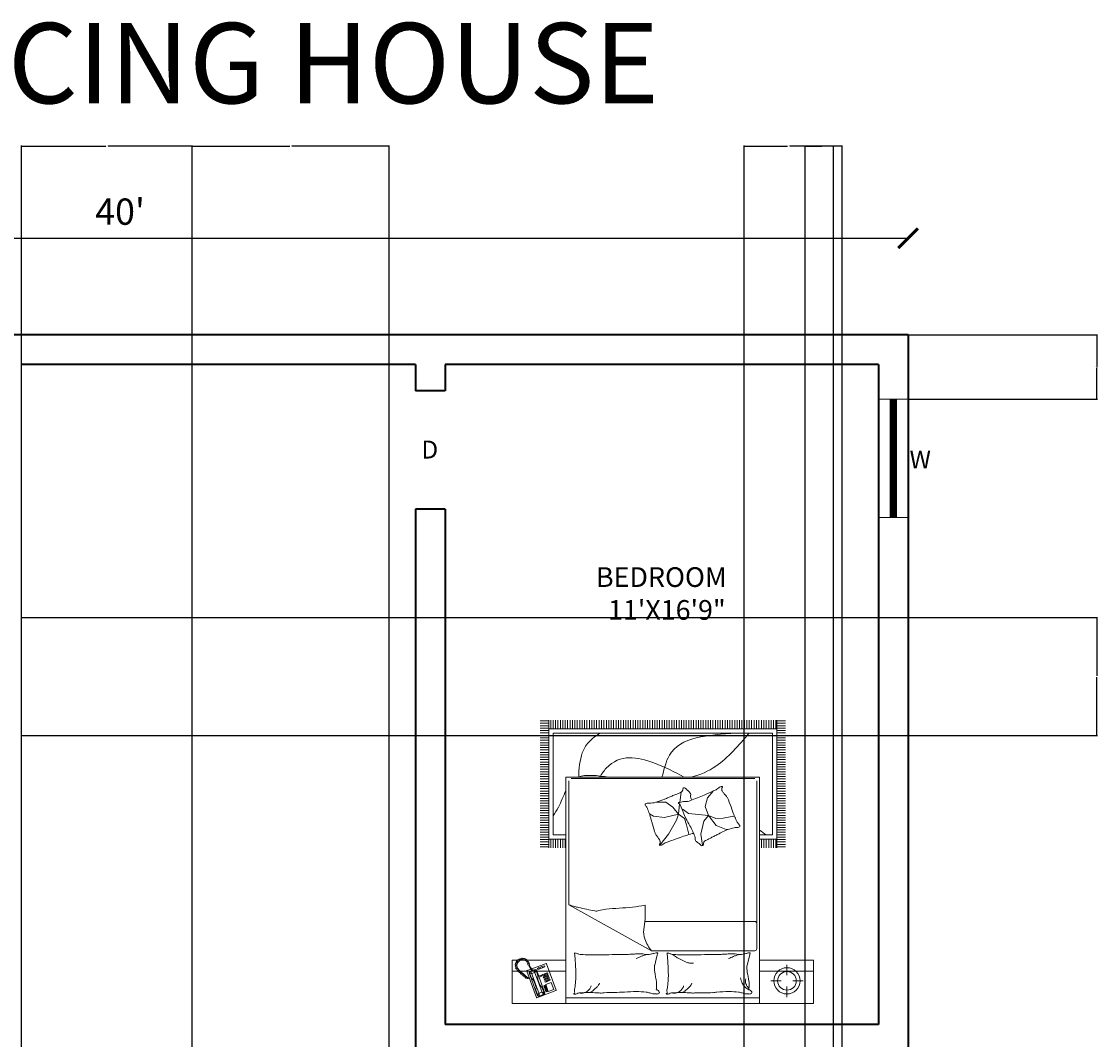
# Model space of a CAD drawing. Units: inches. Extents: x 318 to 927, y -1130 to 13.
# Tile 17 of 17: x 599 to 927, y -297 to 13. Entities that reach past the tile are written whole.
import ezdxf

# ---------------------------------------------------------------- set-up
doc = ezdxf.new("R2010")
doc.units = ezdxf.units.IN
doc.header["$MEASUREMENT"] = 0
for name, color, linetype, lineweight in [('A-ANNO-DIMS', 1, 'Continuous', 18), ('A-ANNO-IDEN', 1, 'Continuous', 13), ('A-ANNO-TEXT', 8, 'Continuous', 25), ('A-AREA-IDEN', 8, 'Continuous', 18), ('A-GLAZ-PATT', 5, 'Continuous', 9), ('wall', 1, 'Continuous', 35), ('win', 5, 'Continuous', 18)]:
    doc.layers.add(name, color=color, linetype=linetype, lineweight=lineweight)
doc.layers.add('furniture', color=50, linetype='Continuous', lineweight=13, transparency=0.8)
doc.styles.add('DIM_FONT', font='SIMPLEX.shx', dxfattribs={"width": 0.8})
doc.styles.get("Standard").update_dxf_attribs({"font": 'arial.ttf'})
doc.dimstyles.get("Standard").update_dxf_attribs({"dimtxt": 0.18, "dimasz": 0.18, "dimexe": 0.18, "dimexo": 0.0625, "dimgap": 0.09, "dimtad": 0, "dimtih": 1, "dimtoh": 1, "dimdec": 1, "dimzin": 0, "dimdsep": 46, "dimlunit": 4, "dimtxsty": 'Standard', "dimcen": 0.09, "dimadec": 0, "dimazin": 0, "dimtfac": 1, "dimtdec": 1, "dimtofl": 0, "dimtmove": 0, "dimatfit": 3, "dimfxl": 1, "dimtolj": 1, "dimtzin": 0, "dimarcsym": 0})

# ---------------------------------------------------------------- blocks, each defined once
blk = doc.blocks.new('A$C4F634EDD')
for p, q in [((0, 2.629), (0, 2.229)), ((0.5, 2.629), (0, 2.629)), ((0.5, 2.629), (2.3, 2.629)), ((0.5, 0.529), (0.5, 2.629)), ((0.5, 2.229), (0.5, 2.629)), ((2.3, 2.629), (2.3, 0.529)), ((2.3, 2.629), (2.8, 2.629)), ((2.3, 2.229), (2.3, 2.629)), ((2.8, 2.629), (2.8, 2.229)), ((0.246, 2.57), (0.246, 2.473)), ((0.5, 2.577), (2.3, 2.577)), ((2.39, 2.507), (2.392, 2.511)), ((2.48, 2.262), (2.39, 2.507)), ((2.392, 2.511), (2.569, 2.577)), ((2.412, 2.501), (2.463, 2.52)), ((2.463, 2.52), (2.487, 2.454)), ((2.484, 2.523), (2.47, 2.518)), ((2.47, 2.518), (2.472, 2.513)), ((2.472, 2.513), (2.486, 2.518)), ((2.488, 2.513), (2.474, 2.507)), ((2.474, 2.507), (2.476, 2.502)), ((2.476, 2.502), (2.49, 2.507)), ((2.492, 2.502), (2.478, 2.497)), ((2.486, 2.518), (2.484, 2.523)), ((2.49, 2.507), (2.488, 2.513)), ((2.494, 2.497), (2.492, 2.502)), ((2.495, 2.533), (2.498, 2.545)), ((2.573, 2.319), (2.495, 2.533)), ((2.498, 2.545), (2.552, 2.564)), ((2.506, 2.545), (2.5, 2.539)), ((2.5, 2.539), (2.501, 2.531)), ((2.501, 2.531), (2.519, 2.484)), ((2.501, 2.531), (2.523, 2.521)), ((2.506, 2.545), (2.549, 2.561)), ((2.524, 2.526), (2.506, 2.545)), ((2.523, 2.521), (2.524, 2.526)), ((2.552, 2.442), (2.523, 2.521)), ((2.548, 2.535), (2.524, 2.526)), ((2.548, 2.535), (2.549, 2.561)), ((2.551, 2.532), (2.548, 2.535)), ((2.549, 2.561), (2.557, 2.56)), ((2.562, 2.554), (2.551, 2.532)), ((2.581, 2.452), (2.551, 2.532)), ((2.552, 2.564), (2.564, 2.558)), ((2.557, 2.56), (2.562, 2.554)), ((2.562, 2.554), (2.579, 2.506)), ((2.564, 2.558), (2.642, 2.346)), ((2.569, 2.577), (2.574, 2.574)), ((2.574, 2.574), (2.664, 2.33)), ((2.579, 2.506), (2.579, 2.496)), ((0.096, 2.42), (0.192, 2.42)), ((0.299, 2.42), (0.396, 2.42)), ((2.436, 2.435), (2.412, 2.501)), ((2.487, 2.454), (2.436, 2.435)), ((2.446, 2.415), (2.456, 2.418)), ((2.45, 2.404), (2.446, 2.415)), ((2.46, 2.408), (2.45, 2.404)), ((2.456, 2.418), (2.46, 2.408)), ((2.463, 2.421), (2.474, 2.425)), ((2.467, 2.41), (2.463, 2.421)), ((2.478, 2.414), (2.467, 2.41)), ((2.471, 2.402), (2.481, 2.405)), ((2.474, 2.391), (2.471, 2.402)), ((2.474, 2.425), (2.478, 2.414)), ((2.478, 2.497), (2.48, 2.491)), ((2.48, 2.491), (2.494, 2.497)), ((2.481, 2.428), (2.492, 2.431)), ((2.485, 2.417), (2.481, 2.428)), ((2.481, 2.405), (2.485, 2.395)), ((2.496, 2.491), (2.482, 2.486)), ((2.482, 2.486), (2.484, 2.481)), ((2.484, 2.481), (2.498, 2.486)), ((2.496, 2.421), (2.485, 2.417)), ((2.5, 2.481), (2.486, 2.475)), ((2.486, 2.475), (2.488, 2.47)), ((2.488, 2.47), (2.502, 2.475)), ((2.488, 2.408), (2.499, 2.412)), ((2.492, 2.397), (2.488, 2.408)), ((2.504, 2.47), (2.49, 2.465)), ((2.49, 2.465), (2.491, 2.46)), ((2.491, 2.46), (2.506, 2.465)), ((2.492, 2.431), (2.496, 2.421)), ((2.503, 2.401), (2.492, 2.397)), ((2.498, 2.486), (2.496, 2.491)), ((2.499, 2.412), (2.503, 2.401)), ((2.502, 2.475), (2.5, 2.481)), ((2.506, 2.465), (2.504, 2.47)), ((2.519, 2.484), (2.526, 2.476)), ((2.526, 2.476), (2.534, 2.469)), ((2.534, 2.469), (2.541, 2.457)), ((2.541, 2.457), (2.547, 2.44)), ((2.559, 2.406), (2.547, 2.44)), ((2.552, 2.442), (2.587, 2.346)), ((2.562, 2.393), (2.559, 2.406)), ((2.579, 2.496), (2.577, 2.485)), ((2.577, 2.485), (2.579, 2.472)), ((2.579, 2.472), (2.586, 2.454)), ((2.581, 2.452), (2.616, 2.356)), ((2.598, 2.42), (2.586, 2.454)), ((2.605, 2.409), (2.598, 2.42)), ((2.613, 2.402), (2.605, 2.409)), ((2.62, 2.394), (2.613, 2.402)), ((0, 2.33), (0.5, 2.33)), ((0.246, 2.366), (0.246, 2.27)), ((2.8, 2.33), (2.3, 2.33)), ((2.453, 2.395), (2.463, 2.399)), ((2.457, 2.384), (2.453, 2.395)), ((2.467, 2.388), (2.457, 2.384)), ((2.46, 2.376), (2.471, 2.379)), ((2.464, 2.365), (2.46, 2.376)), ((2.463, 2.399), (2.467, 2.388)), ((2.475, 2.369), (2.464, 2.365)), ((2.467, 2.356), (2.478, 2.36)), ((2.471, 2.345), (2.467, 2.356)), ((2.471, 2.379), (2.475, 2.369)), ((2.482, 2.349), (2.471, 2.345)), ((2.485, 2.395), (2.474, 2.391)), ((2.478, 2.382), (2.488, 2.386)), ((2.482, 2.371), (2.478, 2.382)), ((2.478, 2.36), (2.482, 2.349)), ((2.492, 2.375), (2.482, 2.371)), ((2.617, 2.309), (2.484, 2.26)), ((2.485, 2.363), (2.495, 2.367)), ((2.489, 2.352), (2.485, 2.363)), ((2.488, 2.386), (2.492, 2.375)), ((2.499, 2.356), (2.489, 2.352)), ((2.495, 2.389), (2.506, 2.392)), ((2.499, 2.378), (2.495, 2.389)), ((2.495, 2.367), (2.499, 2.356)), ((2.51, 2.382), (2.499, 2.378)), ((2.503, 2.369), (2.513, 2.373)), ((2.506, 2.358), (2.503, 2.369)), ((2.506, 2.392), (2.51, 2.382)), ((2.517, 2.362), (2.506, 2.358)), ((2.513, 2.373), (2.517, 2.362)), ((2.536, 2.305), (2.518, 2.299)), ((2.524, 2.377), (2.538, 2.382)), ((2.528, 2.366), (2.524, 2.377)), ((2.542, 2.371), (2.528, 2.366)), ((2.54, 2.294), (2.536, 2.305)), ((2.538, 2.382), (2.542, 2.371)), ((2.561, 2.314), (2.543, 2.308)), ((2.543, 2.308), (2.547, 2.297)), ((2.547, 2.297), (2.565, 2.304)), ((2.56, 2.382), (2.562, 2.393)), ((2.56, 2.372), (2.56, 2.382)), ((2.577, 2.324), (2.56, 2.372)), ((2.565, 2.304), (2.561, 2.314)), ((2.585, 2.313), (2.573, 2.319)), ((2.577, 2.324), (2.587, 2.346)), ((2.582, 2.318), (2.577, 2.324)), ((2.59, 2.317), (2.582, 2.318)), ((2.61, 2.322), (2.585, 2.313)), ((2.587, 2.346), (2.591, 2.343)), ((2.591, 2.343), (2.59, 2.317)), ((2.59, 2.317), (2.61, 2.324)), ((2.615, 2.352), (2.591, 2.343)), ((2.613, 2.331), (2.608, 2.329)), ((2.608, 2.329), (2.614, 2.314)), ((2.619, 2.317), (2.613, 2.331)), ((2.614, 2.314), (2.624, 2.298)), ((2.616, 2.356), (2.615, 2.352)), ((2.615, 2.352), (2.633, 2.332)), ((2.615, 2.326), (2.633, 2.332)), ((2.638, 2.346), (2.616, 2.356)), ((2.637, 2.332), (2.616, 2.324)), ((2.626, 2.307), (2.619, 2.317)), ((2.638, 2.346), (2.62, 2.394)), ((2.662, 2.325), (2.623, 2.311)), ((2.636, 2.292), (2.626, 2.307)), ((2.633, 2.332), (2.638, 2.339)), ((2.642, 2.346), (2.637, 2.332)), ((2.638, 2.339), (2.638, 2.346)), ((2.65, 2.398), (2.64, 2.395)), ((2.642, 2.39), (2.649, 2.391)), ((2.649, 2.391), (2.654, 2.39)), ((2.655, 2.397), (2.65, 2.398)), ((2.654, 2.39), (2.66, 2.388)), ((2.663, 2.392), (2.655, 2.397)), ((2.66, 2.388), (2.663, 2.387)), ((2.664, 2.33), (2.662, 2.325)), ((2.669, 2.394), (2.663, 2.392)), ((2.663, 2.387), (2.666, 2.388)), ((2.666, 2.388), (2.663, 2.383)), ((2.663, 2.383), (2.674, 2.374)), ((2.674, 2.394), (2.669, 2.394)), ((2.676, 2.391), (2.674, 2.394)), ((2.674, 2.38), (2.676, 2.391)), ((2.682, 2.386), (2.674, 2.38)), ((2.674, 2.374), (2.692, 2.359)), ((2.687, 2.381), (2.682, 2.386)), ((2.685, 2.369), (2.687, 2.381)), ((2.695, 2.376), (2.685, 2.369)), ((2.692, 2.359), (2.705, 2.347)), ((2.7, 2.371), (2.695, 2.376)), ((2.695, 2.36), (2.7, 2.371)), ((2.703, 2.368), (2.695, 2.36)), ((2.71, 2.362), (2.703, 2.368)), ((2.705, 2.347), (2.708, 2.348)), ((2.706, 2.351), (2.71, 2.362)), ((2.715, 2.358), (2.706, 2.351)), ((2.708, 2.348), (2.708, 2.344)), ((2.708, 2.344), (2.727, 2.328)), ((2.721, 2.352), (2.715, 2.358)), ((2.72, 2.34), (2.721, 2.352)), ((2.729, 2.347), (2.72, 2.34)), ((2.727, 2.328), (2.751, 2.298)), ((2.735, 2.342), (2.729, 2.347)), ((2.732, 2.33), (2.735, 2.342)), ((2.742, 2.335), (2.732, 2.33)), ((2.741, 2.317), (2.75, 2.325)), ((2.752, 2.322), (2.741, 2.317)), ((2.75, 2.325), (2.742, 2.335)), ((2.757, 2.314), (2.752, 2.322)), ((2.753, 2.304), (2.757, 2.314)), ((2.762, 2.308), (2.753, 2.304)), ((2.767, 2.3), (2.762, 2.308)), ((0, 2.229), (0.5, 2.229)), ((0.595, 2.191), (0.616, 2.274)), ((1.455, 2.191), (1.475, 2.274)), ((2.8, 2.229), (2.3, 2.229)), ((2.484, 2.26), (2.48, 2.262)), ((2.511, 2.296), (2.494, 2.289)), ((2.494, 2.289), (2.498, 2.279)), ((2.498, 2.279), (2.515, 2.285)), ((2.515, 2.285), (2.511, 2.296)), ((2.518, 2.299), (2.522, 2.288)), ((2.522, 2.288), (2.54, 2.294)), ((2.624, 2.298), (2.635, 2.282)), ((2.635, 2.282), (2.638, 2.273)), ((2.641, 2.283), (2.636, 2.292)), ((2.64, 2.271), (2.637, 2.266)), ((2.637, 2.266), (2.64, 2.257)), ((2.638, 2.273), (2.64, 2.271)), ((2.64, 2.257), (2.651, 2.259)), ((2.644, 2.274), (2.641, 2.283)), ((2.651, 2.259), (2.643, 2.249)), ((2.643, 2.249), (2.647, 2.24)), ((2.652, 2.272), (2.644, 2.274)), ((2.647, 2.24), (2.659, 2.243)), ((2.654, 2.263), (2.652, 2.272)), ((2.659, 2.243), (2.652, 2.231)), ((2.652, 2.231), (2.66, 2.225)), ((2.664, 2.241), (2.654, 2.263)), ((2.66, 2.225), (2.67, 2.231)), ((2.684, 2.229), (2.664, 2.241)), ((2.67, 2.231), (2.668, 2.219)), ((2.668, 2.219), (2.676, 2.215)), ((2.676, 2.215), (2.682, 2.224)), ((2.682, 2.224), (2.684, 2.213)), ((2.706, 2.226), (2.684, 2.229)), ((2.684, 2.213), (2.693, 2.212)), ((2.693, 2.212), (2.699, 2.222)), ((2.699, 2.222), (2.702, 2.21)), ((2.702, 2.21), (2.71, 2.21)), ((2.728, 2.232), (2.706, 2.226)), ((2.71, 2.21), (2.711, 2.222)), ((2.711, 2.222), (2.719, 2.214)), ((2.719, 2.214), (2.726, 2.215)), ((2.726, 2.215), (2.724, 2.227)), ((2.724, 2.227), (2.732, 2.216)), ((2.746, 2.248), (2.728, 2.232)), ((2.732, 2.216), (2.739, 2.221)), ((2.739, 2.221), (2.735, 2.231)), ((2.735, 2.231), (2.746, 2.226)), ((2.756, 2.27), (2.746, 2.248)), ((2.751, 2.231), (2.746, 2.242)), ((2.746, 2.242), (2.757, 2.235)), ((2.746, 2.226), (2.751, 2.231)), ((2.751, 2.298), (2.756, 2.27)), ((2.753, 2.25), (2.764, 2.25)), ((2.761, 2.242), (2.753, 2.25)), ((2.757, 2.292), (2.767, 2.3)), ((2.769, 2.29), (2.757, 2.292)), ((2.757, 2.235), (2.761, 2.242)), ((2.759, 2.279), (2.77, 2.283)), ((2.771, 2.273), (2.759, 2.279)), ((2.759, 2.264), (2.771, 2.264)), ((2.768, 2.256), (2.759, 2.264)), ((2.764, 2.25), (2.768, 2.256)), ((2.77, 2.283), (2.769, 2.29)), ((2.771, 2.264), (2.771, 2.273)), ((0.526, 2.121), (0.526, 0.562)), ((1.503, 2.141), (0.546, 2.141)), ((0.588, 2.161), (0.595, 2.191)), ((1.447, 2.161), (1.455, 2.191)), ((1.503, 2.141), (2.272, 1.714)), ((1.576, 1.943), (1.562, 1.848)), ((0.546, 1.868), (1.565, 1.868)), ((1.562, 1.848), (1.564, 1.718)), ((2.272, 0.562), (2.272, 1.714)), ((0.259, 1.175), (0.339, 1.175)), ((0.259, 1.153), (0.339, 1.153)), ((0.259, 1.13), (0.339, 1.13)), ((0.259, 1.108), (0.339, 1.108)), ((0.339, 0), (0.339, 1.185)), ((0.339, 1.105), (0.5, 1.105)), ((0.349, 1.105), (0.349, 1.185)), ((0.371, 1.105), (0.371, 1.185)), ((0.394, 1.105), (0.394, 1.185)), ((0.416, 1.105), (0.416, 1.185)), ((0.439, 1.105), (0.439, 1.185)), ((0.461, 1.105), (0.461, 1.185)), ((0.484, 1.105), (0.484, 1.185)), ((1.031, 1.161), (1.045, 1.058)), ((1.428, 1.161), (1.348, 1.057)), ((2.3, 1.105), (2.459, 1.105)), ((2.306, 1.105), (2.306, 1.185)), ((2.329, 1.105), (2.329, 1.185)), ((2.351, 1.105), (2.351, 1.185)), ((2.374, 1.105), (2.374, 1.185)), ((2.396, 1.105), (2.396, 1.185)), ((2.419, 1.105), (2.419, 1.185)), ((2.441, 1.105), (2.441, 1.185)), ((2.459, 1.185), (2.459, 0)), ((2.459, 1.175), (2.539, 1.175)), ((2.459, 1.153), (2.539, 1.153)), ((2.459, 1.13), (2.539, 1.13)), ((2.459, 1.108), (2.539, 1.108)), ((0.259, 1.085), (0.339, 1.085)), ((0.259, 1.063), (0.339, 1.063)), ((0.259, 1.04), (0.339, 1.04)), ((0.259, 1.018), (0.339, 1.018)), ((0.379, 1.065), (0.5, 1.065)), ((0.379, 0.12), (0.379, 1.065)), ((0.811, 1.015), (0.787, 1.012)), ((0.905, 0.977), (0.811, 1.015)), ((1.045, 1.058), (1.019, 0.936)), ((1.178, 0.97), (1.159, 1.059)), ((1.348, 1.057), (1.273, 0.927)), ((2.3, 1.065), (2.419, 1.065)), ((2.419, 1.065), (2.419, 0.12)), ((2.459, 1.085), (2.539, 1.085)), ((2.459, 1.063), (2.539, 1.063)), ((2.459, 1.04), (2.539, 1.04)), ((2.459, 1.018), (2.539, 1.018)), ((0.259, 0.995), (0.339, 0.995)), ((0.259, 0.973), (0.339, 0.973)), ((0.259, 0.95), (0.339, 0.95)), ((0.259, 0.928), (0.339, 0.928)), ((0.259, 0.905), (0.339, 0.905)), ((0.838, 0.909), (0.74, 0.891)), ((0.907, 0.912), (0.838, 0.909)), ((0.974, 0.884), (0.905, 0.977)), ((0.974, 0.884), (0.907, 0.912)), ((1.019, 0.936), (0.974, 0.884)), ((1.198, 0.913), (1.178, 0.97)), ((1.255, 0.871), (1.198, 0.913)), ((1.273, 0.927), (1.255, 0.871)), ((1.255, 0.871), (1.384, 0.903)), ((1.384, 0.903), (1.487, 0.889)), ((2.459, 0.995), (2.539, 0.995)), ((2.459, 0.973), (2.539, 0.973)), ((2.459, 0.95), (2.539, 0.95)), ((2.459, 0.928), (2.539, 0.928)), ((2.459, 0.905), (2.539, 0.905)), ((0.259, 0.883), (0.339, 0.883)), ((0.259, 0.86), (0.339, 0.86)), ((0.259, 0.838), (0.339, 0.838)), ((0.259, 0.815), (0.339, 0.815)), ((0.74, 0.891), (0.737, 0.885)), ((0.974, 0.884), (1.005, 0.802)), ((0.974, 0.884), (1.16, 0.866)), ((1.005, 0.802), (0.985, 0.719)), ((1.16, 0.866), (1.21, 0.829)), ((1.197, 0.885), (1.22, 0.829)), ((1.21, 0.829), (1.222, 0.821)), ((1.22, 0.829), (1.238, 0.786)), ((1.255, 0.871), (1.244, 0.777)), ((1.255, 0.871), (1.305, 0.808)), ((1.305, 0.808), (1.37, 0.761)), ((1.487, 0.889), (1.523, 0.869)), ((2.459, 0.883), (2.539, 0.883)), ((2.459, 0.86), (2.539, 0.86)), ((2.459, 0.838), (2.539, 0.838)), ((2.459, 0.815), (2.539, 0.815)), ((0.259, 0.793), (0.339, 0.793)), ((0.259, 0.77), (0.339, 0.77)), ((0.259, 0.748), (0.339, 0.748)), ((0.259, 0.725), (0.339, 0.725)), ((0.259, 0.703), (0.339, 0.703)), ((0.985, 0.719), (0.931, 0.657)), ((1.242, 0.763), (1.23, 0.668)), ((1.37, 0.761), (1.463, 0.761)), ((2.459, 0.793), (2.539, 0.793)), ((2.459, 0.77), (2.539, 0.77)), ((2.459, 0.748), (2.539, 0.748)), ((2.459, 0.725), (2.539, 0.725)), ((2.459, 0.703), (2.539, 0.703)), ((0.259, 0.68), (0.339, 0.68)), ((0.259, 0.658), (0.339, 0.658)), ((0.259, 0.635), (0.339, 0.635)), ((0.259, 0.613), (0.339, 0.613)), ((2.459, 0.68), (2.539, 0.68)), ((2.459, 0.658), (2.539, 0.658)), ((2.459, 0.635), (2.539, 0.635)), ((2.459, 0.613), (2.539, 0.613)), ((0.259, 0.59), (0.339, 0.59)), ((0.259, 0.568), (0.339, 0.568)), ((0.259, 0.545), (0.339, 0.545)), ((0.259, 0.523), (0.339, 0.523)), ((0.259, 0.5), (0.339, 0.5)), ((2.3, 0.529), (0.5, 0.529)), ((0.546, 0.542), (2.252, 0.542)), ((2.459, 0.59), (2.539, 0.59)), ((2.459, 0.568), (2.539, 0.568)), ((2.459, 0.545), (2.539, 0.545)), ((2.459, 0.523), (2.539, 0.523)), ((2.459, 0.5), (2.539, 0.5)), ((0.259, 0.478), (0.339, 0.478)), ((0.259, 0.455), (0.339, 0.455)), ((0.259, 0.433), (0.339, 0.433)), ((0.259, 0.41), (0.339, 0.41)), ((2.459, 0.478), (2.539, 0.478)), ((2.459, 0.455), (2.539, 0.455)), ((2.459, 0.433), (2.539, 0.433)), ((2.459, 0.41), (2.539, 0.41)), ((0.259, 0.388), (0.339, 0.388)), ((0.259, 0.365), (0.339, 0.365)), ((0.259, 0.343), (0.339, 0.343)), ((0.259, 0.32), (0.339, 0.32)), ((2.459, 0.388), (2.539, 0.388)), ((2.459, 0.365), (2.539, 0.365)), ((2.459, 0.343), (2.539, 0.343)), ((2.459, 0.32), (2.539, 0.32)), ((0.259, 0.298), (0.339, 0.298)), ((0.259, 0.275), (0.339, 0.275)), ((0.259, 0.253), (0.339, 0.253)), ((0.259, 0.23), (0.339, 0.23)), ((0.259, 0.208), (0.339, 0.208)), ((2.459, 0.298), (2.539, 0.298)), ((2.459, 0.275), (2.539, 0.275)), ((2.459, 0.253), (2.539, 0.253)), ((2.459, 0.23), (2.539, 0.23)), ((2.459, 0.208), (2.539, 0.208)), ((0.259, 0.185), (0.339, 0.185)), ((0.259, 0.163), (0.339, 0.163)), ((0.259, 0.14), (0.339, 0.14)), ((0.259, 0.118), (0.339, 0.118)), ((2.419, 0.12), (0.379, 0.12)), ((2.459, 0.185), (2.539, 0.185)), ((2.459, 0.163), (2.539, 0.163)), ((2.459, 0.14), (2.539, 0.14)), ((2.459, 0.118), (2.539, 0.118)), ((0.259, 0.095), (0.339, 0.095)), ((0.259, 0.073), (0.339, 0.073)), ((0.259, 0.05), (0.339, 0.05)), ((0.259, 0.028), (0.339, 0.028)), ((0.259, 0.005), (0.339, 0.005)), ((2.459, 0.08), (0.339, 0.08)), ((0.349, 0), (0.349, 0.08)), ((0.371, 0), (0.371, 0.08)), ((0.394, 0), (0.394, 0.08)), ((0.416, 0), (0.416, 0.08)), ((0.439, 0), (0.439, 0.08)), ((0.461, 0), (0.461, 0.08)), ((0.484, 0), (0.484, 0.08)), ((0.506, 0), (0.506, 0.08)), ((0.529, 0), (0.529, 0.08)), ((0.551, 0), (0.551, 0.08)), ((0.574, 0), (0.574, 0.08)), ((0.596, 0), (0.596, 0.08)), ((0.619, 0), (0.619, 0.08)), ((0.641, 0), (0.641, 0.08)), ((0.664, 0), (0.664, 0.08)), ((0.686, 0), (0.686, 0.08)), ((0.709, 0), (0.709, 0.08)), ((0.731, 0), (0.731, 0.08)), ((0.754, 0), (0.754, 0.08)), ((0.776, 0), (0.776, 0.08)), ((0.799, 0), (0.799, 0.08)), ((0.821, 0), (0.821, 0.08)), ((0.844, 0), (0.844, 0.08)), ((0.866, 0), (0.866, 0.08)), ((0.889, 0), (0.889, 0.08)), ((0.911, 0), (0.911, 0.08)), ((0.934, 0), (0.934, 0.08)), ((0.956, 0), (0.956, 0.08)), ((0.979, 0), (0.979, 0.08)), ((1.001, 0), (1.001, 0.08)), ((1.024, 0), (1.024, 0.08)), ((1.046, 0), (1.046, 0.08)), ((1.069, 0), (1.069, 0.08)), ((1.091, 0), (1.091, 0.08)), ((1.114, 0), (1.114, 0.08)), ((1.136, 0), (1.136, 0.08)), ((1.159, 0), (1.159, 0.08)), ((1.181, 0), (1.181, 0.08)), ((1.204, 0), (1.204, 0.08)), ((1.226, 0), (1.226, 0.08)), ((1.249, 0), (1.249, 0.08)), ((1.271, 0), (1.271, 0.08)), ((1.294, 0), (1.294, 0.08)), ((1.316, 0), (1.316, 0.08)), ((1.339, 0), (1.339, 0.08)), ((1.361, 0), (1.361, 0.08)), ((1.384, 0), (1.384, 0.08)), ((1.406, 0), (1.406, 0.08)), ((1.429, 0), (1.429, 0.08)), ((1.451, 0), (1.451, 0.08)), ((1.474, 0), (1.474, 0.08)), ((1.496, 0), (1.496, 0.08)), ((1.519, 0), (1.519, 0.08)), ((1.541, 0), (1.541, 0.08)), ((1.564, 0), (1.564, 0.08)), ((1.586, 0), (1.586, 0.08)), ((1.609, 0), (1.609, 0.08)), ((1.631, 0), (1.631, 0.08)), ((1.654, 0), (1.654, 0.08)), ((1.676, 0), (1.676, 0.08)), ((1.699, 0), (1.699, 0.08)), ((1.721, 0), (1.721, 0.08)), ((1.744, 0), (1.744, 0.08)), ((1.766, 0), (1.766, 0.08)), ((1.789, 0), (1.789, 0.08)), ((1.811, 0), (1.811, 0.08)), ((1.834, 0), (1.834, 0.08)), ((1.856, 0), (1.856, 0.08)), ((1.879, 0), (1.879, 0.08)), ((1.901, 0), (1.901, 0.08)), ((1.924, 0), (1.924, 0.08)), ((1.946, 0), (1.946, 0.08)), ((1.969, 0), (1.969, 0.08)), ((1.991, 0), (1.991, 0.08)), ((2.014, 0), (2.014, 0.08)), ((2.036, 0), (2.036, 0.08)), ((2.059, 0), (2.059, 0.08)), ((2.081, 0), (2.081, 0.08)), ((2.104, 0), (2.104, 0.08)), ((2.126, 0), (2.126, 0.08)), ((2.149, 0), (2.149, 0.08)), ((2.171, 0), (2.171, 0.08)), ((2.194, 0), (2.194, 0.08)), ((2.216, 0), (2.216, 0.08)), ((2.239, 0), (2.239, 0.08)), ((2.261, 0), (2.261, 0.08)), ((2.284, 0), (2.284, 0.08)), ((2.306, 0), (2.306, 0.08)), ((2.329, 0), (2.329, 0.08)), ((2.351, 0), (2.351, 0.08)), ((2.374, 0), (2.374, 0.08)), ((2.396, 0), (2.396, 0.08)), ((2.419, 0), (2.419, 0.08)), ((2.441, 0), (2.441, 0.08)), ((2.459, 0.095), (2.539, 0.095)), ((2.459, 0.073), (2.539, 0.073)), ((2.459, 0.05), (2.539, 0.05)), ((2.459, 0.028), (2.539, 0.028)), ((2.459, 0.005), (2.539, 0.005))]:
    blk.add_line(p, q)
for radius in [0.122, 0.0865]:
    blk.add_circle((0.246, 2.42), radius)
for centre, radius, start, end in [((0.585, 2.527), 0.0131, 101.2724, 206.5805), ((0.604, 2.537), 0.0342, 206.5805, 265.5998), ((0.6, 2.452), 0.0904, 90, 101.2724), ((1.09, 2.45), 0.492, 173.7676, 180), ((0.6, 2.381), 0.161, 81.5628, 90), ((0.537, 2.378), 0.14, 45.0976, 62.7964), ((0.579, 2.239), 0.305, 74.256, 81.5628), ((0.727, 2.765), 0.242, 254.256, 262.4531), ((0.785, 3.202), 0.683, 262.4531, 270), ((0.785, 3.568), 1.049, 270, 276.0867), ((0.84, 3.051), 0.529, 276.0867, 280.1899), ((1.16, -8.135), 10.667, 90.3015, 91.2158), ((1.117, 2.243), 0.29, 85.1982, 92.5386), ((1.214, 3.402), 0.873, 265.1982, 269.4243), ((1.432, 2.203), 0.392, 128.3886, 133.8115), ((1.236, 2.45), 0.0768, 117.2396, 128.3886), ((1.308, 2.31), 0.234, 110.8603, 117.2396), ((1.22, 4.023), 1.494, 269.4243, 271.9079), ((1.3, 2.436), 0.0992, 126.0864, 143.8234), ((1.3, 2.436), 0.0992, 105.9352, 126.0864), ((1.243, 3.35), 0.821, 271.9079, 275.2592), ((1.3, 2.436), 0.0992, 85.7841, 105.9352), ((1.313, 2.586), 0.0539, 275.2592, 300.6513), ((1.355, 2.515), 0.0289, 85.6975, 120.6513), ((1.356, 2.519), 0.0251, 68.2117, 85.6975), ((1.374, 2.529), 0.0156, 158.0096, 201.421), ((1.118, 2.541), 0.246, 347.8905, 351.8665), ((1.363, 2.533), 0.00428, 78.1069, 158.0096), ((1.329, 2.511), 0.0328, 351.8665, 21.421), ((1.365, 2.539), 0.00232, 258.1069, 19.564), ((1.364, 2.539), 0.00342, 19.564, 68.2117), ((1.444, 2.527), 0.0131, 101.2724, 206.5805), ((1.463, 2.537), 0.0342, 206.5805, 265.5998), ((1.459, 2.452), 0.0904, 90, 101.2724), ((1.949, 2.45), 0.492, 173.7676, 180), ((1.459, 2.381), 0.161, 81.5628, 90), ((1.438, 2.239), 0.305, 74.256, 81.5628), ((1.586, 2.765), 0.242, 254.256, 262.4531), ((1.644, 3.202), 0.683, 262.4531, 270), ((1.644, 3.568), 1.049, 270, 276.0867), ((1.479, 15.488), 12.966, 271.2243, 272.0532), ((1.97, 2.381), 0.152, 92.5386, 100.1899), ((1.976, 2.243), 0.29, 85.1982, 92.5386), ((2.073, 3.402), 0.873, 265.1982, 269.4243), ((2.291, 2.203), 0.392, 128.3886, 133.8115), ((2.095, 2.45), 0.0768, 117.2396, 128.3886), ((2.167, 2.31), 0.234, 110.8603, 117.2396), ((2.08, 4.023), 1.494, 269.4243, 271.9079), ((2.159, 2.436), 0.0992, 126.0864, 143.8234), ((2.159, 2.436), 0.0992, 105.9352, 126.0864), ((2.102, 3.35), 0.821, 271.9079, 275.2592), ((2.159, 2.436), 0.0992, 85.7841, 105.9352), ((2.172, 2.586), 0.0539, 275.2592, 300.6513), ((2.215, 2.515), 0.0289, 85.6975, 120.6513), ((2.215, 2.519), 0.0251, 68.2117, 85.6975), ((2.233, 2.529), 0.0156, 158.0096, 201.421), ((1.977, 2.541), 0.246, 347.8905, 351.8665), ((2.223, 2.533), 0.00428, 78.1069, 158.0096), ((2.188, 2.511), 0.0328, 351.8665, 21.421), ((2.224, 2.539), 0.00232, 258.1069, 19.564), ((2.223, 2.539), 0.00342, 19.564, 68.2117), ((0.802, 2.45), 0.204, 180, 189.6844), ((0.546, 2.414), 0.0899, 41.4429, 53.7359), ((1.47, 2.564), 0.882, 189.6844, 192.1984), ((0.574, 2.439), 0.0526, 25.3551, 41.4429), ((0.485, 2.397), 0.151, 21.8149, 25.3551), ((0.435, 2.376), 0.206, 18.7799, 21.8149), ((0.576, 2.425), 0.0562, 0, 18.7799), ((0.541, 2.425), 0.0915, 345.3149, 0), ((0.537, 2.378), 0.14, 27.3988, 45.0976), ((0.537, 2.378), 0.14, 16.515, 27.3988), ((0.537, 2.378), 0.14, 5.6311, 16.515), ((1.313, 2.363), 0.2, 151.6832, 156.9972), ((1.18, 2.434), 0.0493, 140.9651, 151.6832), ((1.317, 2.323), 0.225, 133.8115, 140.9651), ((1.3, 2.436), 0.0992, 143.8234, 161.5603), ((2.027, 2.366), 0.679, 176.6313, 181.6331), ((2.261, 2.353), 0.913, 172.3191, 176.6313), ((1.552, 2.448), 0.198, 167.8905, 172.3191), ((1.661, 2.45), 0.204, 180, 189.6844), ((2.33, 2.564), 0.882, 189.6844, 192.1984), ((2.172, 2.363), 0.2, 151.6832, 156.9972), ((2.039, 2.434), 0.0493, 140.9651, 151.6832), ((2.176, 2.323), 0.225, 133.8115, 140.9651), ((2.159, 2.436), 0.0992, 143.8234, 161.5603), ((2.886, 2.366), 0.679, 176.6313, 181.6331), ((3.12, 2.353), 0.913, 172.3191, 176.6313), ((2.411, 2.448), 0.198, 167.8905, 172.3191), ((0.298, 2.31), 0.317, 8.0051, 12.1984), ((-0.04, 2.263), 0.659, 2.6649, 8.0051), ((2.713, 2.386), 1.365, 181.6331, 183.055), ((14.966, 3.04), 13.636, 183.055, 183.5049), ((1.157, 2.31), 0.317, 8.0051, 12.1984), ((0.819, 2.263), 0.659, 2.6649, 8.0051), ((3.572, 2.386), 1.365, 181.6331, 183.055), ((15.825, 3.04), 13.636, 183.055, 183.5049), ((0.55, 2.29), 0.0677, 345.9548, 2.6649), ((0.473, 2.881), 0.739, 291.6577, 293.4844), ((0.473, 2.881), 0.739, 293.4844, 295.3111), ((1.13, 1.983), 0.272, 85.9172, 93.5552), ((1.146, 2.197), 0.058, 69.3257, 85.9172), ((0.987, 1.777), 0.507, 65.6735, 69.3257), ((0.606, 0.934), 1.432, 63.5015, 65.6735), ((1.105, 1.936), 0.313, 57.865, 63.5015), ((1.676, 2.226), 0.321, 183.5049, 189.9984), ((1.41, 2.29), 0.0677, 345.9548, 2.6649), ((1.332, 2.881), 0.739, 291.6577, 293.4844), ((1.332, 2.881), 0.739, 293.4844, 295.3111), ((2.535, 2.226), 0.321, 183.5049, 189.9984), ((0.546, 2.121), 0.02, 90, 180), ((0.589, 2.161), 0.000917, 165.9551, 274.0829), ((0.57, 2.43), 0.271, 274.0829, 279.4841), ((0.576, 2.39), 0.23, 279.4841, 287.3864), ((0.681, 2.056), 0.12, 96.4341, 107.3864), ((0.684, 2.03), 0.146, 78.4414, 96.4341), ((0.473, 2.881), 0.739, 287.1982, 289.428), ((0.759, 2.398), 0.23, 258.4414, 272.7491), ((0.473, 2.881), 0.739, 289.428, 291.6577), ((0.703, 3.572), 1.405, 272.7491, 274.6176), ((0.914, 0.959), 1.216, 92.6096, 94.6176), ((1.25, -19.84), 22.018, 90.3791, 91.0196), ((1.201, -3.54), 5.719, 89.7135, 90.9704), ((1.224, 1.014), 1.164, 86.426, 89.7135), ((0.884, 1.584), 0.729, 54.1737, 57.865), ((1.287, 2.03), 0.146, 77.131, 86.426), ((1.31, 2.128), 0.0453, 62.7159, 77.131), ((1.366, 2.237), 0.0767, 242.7159, 253.7788), ((1.369, 2.247), 0.0875, 253.7788, 262.8796), ((1.358, 2.162), 0.00132, 262.8796, 343.3022), ((1.341, 2.167), 0.0193, 343.3022, 9.9984), ((1.448, 2.161), 0.000917, 165.9551, 274.0829), ((1.429, 2.43), 0.271, 274.0829, 279.4841), ((1.436, 2.39), 0.23, 279.4841, 287.3864), ((1.215, 1.902), 0.375, 20.1488, 39.6445), ((1.54, 2.056), 0.12, 96.4341, 107.3864), ((1.543, 2.03), 0.146, 78.4414, 96.4341), ((1.332, 2.881), 0.739, 287.1982, 289.428), ((1.618, 2.398), 0.23, 258.4414, 272.7491), ((1.332, 2.881), 0.739, 289.428, 291.6577), ((1.562, 3.572), 1.405, 272.7491, 274.6176), ((1.773, 0.959), 1.216, 92.6096, 94.6176), ((2.109, -19.84), 22.018, 90.3791, 91.0196), ((2.06, -3.54), 5.719, 89.7135, 90.9704), ((2.083, 1.014), 1.164, 86.426, 89.7135), ((2.147, 2.03), 0.146, 77.131, 86.426), ((2.169, 2.128), 0.0453, 62.7159, 77.131), ((2.225, 2.237), 0.0767, 242.7159, 253.7788), ((2.228, 2.247), 0.0875, 253.7788, 262.8796), ((2.217, 2.162), 0.00132, 262.8796, 343.3022), ((2.2, 2.167), 0.0193, 343.3022, 9.9984), ((1.398, 1.969), 0.18, 351.8644, 20.1488), ((0.546, 1.888), 0.02, 180, 270), ((1.058, 5.464), 3.78, 277.692, 279.495), ((0.61, 18.053), 16.352, 273.757, 274.6239), ((1.419, 4.217), 2.516, 281.6741, 283.1904), ((2.038, 1.579), 0.194, 97.7304, 103.1904), ((2.019, 1.714), 0.0581, 79.2724, 97.7304), ((1.274, -2.223), 4.065, 77.0745, 79.2724), ((2.036, 1.098), 0.657, 74.0648, 77.0745), ((1.713, -0.034), 1.835, 72.2636, 74.0648), ((-0.417, 3.87), 3.097, 296.4147, 297.2902), ((0.986, 1.149), 0.0359, 297.2902, 3.2455), ((1.035, 1.152), 0.0127, 51.1864, 183.2455), ((0.999, 1.108), 0.0697, 45.8726, 51.1864), ((1.079, 1.19), 0.0452, 225.8726, 232.4713), ((1.285, 1.458), 0.383, 232.4713, 233.7837), ((0.668, 0.616), 0.66, 52.7849, 53.7837), ((0.936, 0.969), 0.218, 46.4776, 52.7849), ((1.033, 1.071), 0.0774, 35.8936, 46.4776), ((1.077, 1.103), 0.0226, 351.9508, 35.8936), ((-0.411, 5.908), 5.094, 289.0836, 290.1287), ((1.054, 1.911), 0.837, 290.1287, 292.7069), ((1.347, 1.212), 0.0792, 292.7069, 308.5854), ((1.434, 1.103), 0.0601, 110.3452, 128.5854), ((1.425, 1.126), 0.0352, 86.0516, 110.3452), ((1.5, 1.128), 0.0771, 169.5926, 177.2714), ((1.438, 1.131), 0.0153, 177.2714, 194.5709), ((1.461, 1.137), 0.0393, 194.5709, 206.8179), ((1.438, 1.14), 0.0142, 126.5792, 169.5926), ((1.74, 1.278), 0.352, 206.8179, 210.9056), ((1.427, 1.157), 0.00443, 13.2808, 86.0516), ((1.425, 1.156), 0.0063, 306.5792, 13.2808), ((0.642, 1.417), 0.43, 282.6252, 290.7486), ((0.574, 1.598), 0.624, 290.7486, 297.4921), ((-1.834, 6.224), 5.838, 297.4921, 297.8482), ((3.744, -4.334), 6.102, 117.4999, 117.8482), ((1.857, -0.71), 2.016, 116.4147, 117.4999), ((1.145, 1.093), 0.0458, 171.9508, 202.4162), ((2.032, 1.459), 1.005, 202.4162, 205.0529), ((1.092, 1.164), 0.117, 280.7366, 286.6085), ((2.649, 1.748), 1.687, 205.0529, 207.0884), ((0.227, 4.066), 3.145, 286.6085, 289.0836), ((1.605, 1.197), 0.194, 210.9056, 219.7005), ((1.393, 1.022), 0.081, 26.0735, 39.7005), ((1.289, 0.971), 0.197, 17.8396, 26.0735), ((-0.43, 0.417), 2.003, 15.2625, 17.8396), ((0.689, 0.983), 0.0058, 121.6917, 179.0386), ((0.7, 0.983), 0.0168, 179.0386, 229.4914), ((0.713, 0.945), 0.0509, 103.0402, 121.6917), ((0.64, 0.913), 0.0755, 26.3332, 49.4914), ((0.715, 0.936), 0.0599, 86.6119, 103.0402), ((-1.678, -0.234), 2.662, 25.1732, 26.3332), ((0.722, 1.059), 0.063, 266.6119, 282.6252), ((2.541, 1.692), 1.565, 207.0884, 209.936), ((0.999, 0.804), 0.214, 22.2355, 29.936), ((-0.088, 0.511), 1.648, 13.841, 15.2625), ((2.042, 1.036), 0.545, 193.841, 196.3122), ((0.569, 0.821), 0.18, 20.7081, 25.1732), ((0.227, 0.692), 0.545, 18.2369, 20.7081), ((2.31, 1.379), 1.648, 198.2369, 199.6584), ((2.644, 1.498), 2.003, 199.6584, 202.2355), ((1.691, 0.933), 0.18, 196.3122, 200.7773), ((4.012, 1.813), 2.662, 200.7773, 201.9373), ((1.612, 0.847), 0.0755, 201.9373, 225.0955), ((0.972, 0.814), 0.197, 202.2355, 210.4694), ((0.873, 0.756), 0.081, 210.4694, 224.0964), ((2.269, -2.19), 3.145, 111.0043, 113.4795), ((0.183, 0.409), 1.005, 18.0203, 19.3448), ((1.096, 0.706), 0.0458, 347.5549, 18.0203), ((1.183, 0.637), 0.117, 98.1216, 111.0043), ((1.176, 0.687), 0.0663, 85.4882, 98.1216), ((1.187, 0.824), 0.0712, 265.4882, 277.6784), ((1.173, 0.931), 0.179, 277.6784, 284.8807), ((1.269, 0.569), 0.195, 97.9822, 104.8807), ((1.259, 0.794), 0.0231, 202.2355, 252.8133), ((1.246, 0.729), 0.034, 85.7407, 97.9822), ((1.25, 0.772), 0.0092, 265.7407, 289.3799), ((1.251, 0.768), 0.00467, 289.3799, 72.8133), ((0.523, 2.558), 2.016, 292.0188, 293.104), ((-1.08, 6.316), 6.102, 293.104, 293.4523), ((3.672, -4.638), 5.838, 113.0962, 113.4523), ((1.627, 0.159), 0.624, 106.3527, 113.0962), ((1.572, 0.345), 0.43, 98.2293, 106.3527), ((1.52, 0.708), 0.063, 82.216, 98.2293), ((1.536, 0.83), 0.0599, 262.216, 278.6443), ((1.538, 0.821), 0.0509, 278.6443, 297.2959), ((1.547, 0.782), 0.0168, 354.6428, 45.0955), ((1.558, 0.781), 0.0058, 297.2959, 354.6428), ((0.675, 0.564), 0.194, 35.3015, 44.0964), ((0.546, 0.473), 0.352, 31.2138, 35.3015), ((0.851, 0.619), 0.0063, 130.9751, 197.6767), ((0.849, 0.618), 0.00443, 197.6767, 270.4475), ((0.837, 0.635), 0.0142, 310.9751, 353.9885), ((0.814, 0.635), 0.0393, 18.9668, 31.2138), ((0.849, 0.649), 0.0352, 270.4475, 294.7411), ((0.836, 0.643), 0.0153, 1.6673, 18.9668), ((0.775, 0.641), 0.0771, 353.9885, 1.6673), ((0.838, 0.672), 0.0601, 294.7411, 312.9813), ((0.933, 0.57), 0.0792, 117.1028, 132.9813), ((1.278, -0.105), 0.837, 114.5246, 117.1028), ((3.046, -3.978), 5.094, 113.4795, 114.5246), ((1.162, 0.691), 0.0226, 167.5549, 211.4977), ((1.209, 0.72), 0.0774, 211.4977, 222.0817), ((1.313, 0.814), 0.218, 222.0817, 228.389), ((1.607, 1.145), 0.66, 228.389, 229.3878), ((0.928, 0.353), 0.383, 48.0754, 49.3878), ((1.154, 0.604), 0.0452, 41.4767, 48.0754), ((1.24, 0.68), 0.0697, 221.4767, 226.7905), ((1.201, 0.639), 0.0127, 226.7905, 358.8496), ((1.249, 0.638), 0.0359, 112.8944, 178.8496), ((2.44, -2.182), 3.097, 112.0188, 112.8944)]:
    blk.add_arc(centre, radius, start, end)
for points in [[(0.439, 1.065), (0.46, 1.05), (0.48, 1.035), (0.5, 1.02)], [(1.9, 0.529), (2.006, 0.514), (2.113, 0.498), (2.189, 0.529)]]:
    blk.add_open_spline(points, degree=3)
for points, knots in [([(2.3, 0.653), (2.324, 0.703), (2.355, 0.791), (2.402, 0.861), (2.419, 0.887)], [1893.525221, 1893.525221, 1893.525221, 1893.525221, 2051.902476, 2146.74457, 2146.74457, 2146.74457, 2146.74457]), ([(0.599, 0.12), (0.696, 0.234), (0.852, 0.419), (1.054, 0.507), (1.136, 0.529)], [0, 0, 0, 0, 432.822832, 701.445452, 701.445452, 701.445452, 701.445452]), ([(0.719, 0.12), (0.979, 0.136), (1.326, 0.158), (1.387, 0.457), (1.408, 0.529)], [0, 0, 0, 0, 653.160442, 870.050857, 870.050857, 870.050857, 870.050857]), ([(1.202, 0.529), (1.289, 0.479), (1.514, 0.368), (1.826, 0.299), (1.968, 0.499), (1.987, 0.529)], [936.534237, 936.534237, 936.534237, 936.534237, 1243.285375, 1683.261222, 1758.254386, 1758.254386, 1758.254386, 1758.254386]), ([(2.18, 0.529), (2.18, 0.452), (2.155, 0.237), (2.049, 0.164), (1.985, 0.12)], [2202.034493, 2202.034493, 2202.034493, 2202.034493, 2357.807635, 2594.446174, 2594.446174, 2594.446174, 2594.446174])]:
    blk.add_open_spline(points, degree=3, knots=knots)
at = {"style": 'DIM_FONT', "width": 0.8, "flags": 9}
for tag, p in [('YSIZE', (0.5, 2.629)), ('XSIZE', (0.5, 2.629)), ('XSIZE', (2.298, 2.629)), ('YSIZE', (2.298, 2.629))]:
    blk.add_attdef(tag, p, '', height=0.0005, dxfattribs=at)
blk = doc.blocks.new('_ArchTick')
at = {"color": 0, "linetype": 'ByBlock', "const_width": 0.15}
blk.add_lwpolyline([(-0.5, -0.5), (0.5, 0.5)], dxfattribs=at)
blk = doc.blocks.new('*D3')
at = {"layer": 'A-ANNO-DIMS', "color": 0, "lineweight": -2, "transparency": 16777216}
blk.add_line((388.89, -53.46), (868.89, -53.46), dxfattribs=at)
at = {"layer": 'Defpoints', "color": 0, "transparency": 16777216}
for p in [(868.89, -53.46), (388.89, -82.91), (868.89, -82.91)]:
    blk.add_point(p, dxfattribs=at)
at = {"layer": 'A-ANNO-DIMS', "color": 0, "lineweight": -2, "transparency": 16777216, "xscale": 6, "yscale": 6, "zscale": 6, "rotation": 180}
blk.add_blockref('_ArchTick', (388.89, -53.46), dxfattribs=at)
at = {"layer": 'A-ANNO-DIMS', "color": 0, "lineweight": -2, "transparency": 16777216, "xscale": 6, "yscale": 6, "zscale": 6}
blk.add_blockref('_ArchTick', (868.89, -53.46), dxfattribs=at)
at = {"layer": 'A-ANNO-DIMS', "color": 0, "transparency": 16777216, "insert": (628.89, -45.37), "char_height": 8, "attachment_point": 5}
blk.add_mtext("\\A1;40'", dxfattribs=at)
blk = doc.blocks.new('WIN-36IN')
for p, q in [((0, 36), (9, 36)), ((3.5, 36), (3.5, 0)), ((5.5, 36), (5.5, 0)), ((0, 0), (9, 0))]:
    blk.add_line(p, q)
blk = doc.blocks.new('*D28')
at = {"layer": 'A-ANNO-DIMS', "color": 0, "lineweight": -2, "transparency": 16777216}
for p, q in [((650.89, -1033.85), (650.89, -25.23)), ((651.07, -25.41), (680.57, -25.41)), ((710.71, -25.41), (681.22, -25.41)), ((710.89, -1033.85), (710.89, -25.23))]:
    blk.add_line(p, q, dxfattribs=at)
at = {"layer": 'A-ANNO-DIMS', "color": 0, "transparency": 16777216}
for points in [[(651.07, -25.38), (651.07, -25.44), (650.89, -25.41)], [(710.71, -25.38), (710.71, -25.44), (710.89, -25.41)]]:
    blk.add_solid(points, dxfattribs=at)
at = {"layer": 'Defpoints', "color": 0, "transparency": 16777216}
for p in [(710.89, -25.41), (650.89, -1033.91), (710.89, -1033.91)]:
    blk.add_point(p, dxfattribs=at)
at = {"layer": 'A-ANNO-DIMS', "color": 0, "transparency": 16777216, "insert": (680.89, -25.41), "char_height": 0.18, "attachment_point": 5}
blk.add_mtext('\\A1;5\'-0"', dxfattribs=at)
blk = doc.blocks.new('*D29')
at = {"layer": 'A-ANNO-DIMS', "color": 0, "lineweight": -2, "transparency": 16777216}
for p, q in [((598.89, -1033.85), (598.89, -25.23)), ((599.07, -25.41), (624.56, -25.41)), ((650.71, -25.41), (625.23, -25.41)), ((650.89, -1033.85), (650.89, -25.23))]:
    blk.add_line(p, q, dxfattribs=at)
at = {"layer": 'A-ANNO-DIMS', "color": 0, "transparency": 16777216}
for points in [[(599.07, -25.38), (599.07, -25.44), (598.89, -25.41)], [(650.71, -25.38), (650.71, -25.44), (650.89, -25.41)]]:
    blk.add_solid(points, dxfattribs=at)
at = {"layer": 'Defpoints', "color": 0, "transparency": 16777216}
for p in [(650.89, -25.41), (598.89, -1033.91), (650.89, -1033.91)]:
    blk.add_point(p, dxfattribs=at)
at = {"layer": 'A-ANNO-DIMS', "color": 0, "transparency": 16777216, "insert": (624.89, -25.41), "char_height": 0.18, "attachment_point": 5}
blk.add_mtext('\\A1;4\'-4"', dxfattribs=at)
blk = doc.blocks.new('*D31')
at = {"layer": 'A-ANNO-DIMS', "color": 0, "lineweight": -2, "transparency": 16777216}
for p, q in [((598.96, -168.91), (926.57, -168.91)), ((926.39, -169.09), (926.39, -186.73)), ((926.39, -204.73), (926.39, -187.09)), ((598.96, -204.91), (926.57, -204.91))]:
    blk.add_line(p, q, dxfattribs=at)
at = {"layer": 'A-ANNO-DIMS', "color": 0, "transparency": 16777216}
for points in [[(926.36, -169.09), (926.42, -169.09), (926.39, -168.91)], [(926.36, -204.73), (926.42, -204.73), (926.39, -204.91)]]:
    blk.add_solid(points, dxfattribs=at)
at = {"layer": 'Defpoints', "color": 0, "transparency": 16777216}
for p in [(598.89, -168.91), (598.89, -204.91), (926.39, -204.91)]:
    blk.add_point(p, dxfattribs=at)
at = {"layer": 'A-ANNO-DIMS', "color": 0, "transparency": 16777216, "insert": (926.39, -186.91), "char_height": 0.18, "attachment_point": 5}
blk.add_mtext('\\A1;3\'-0"', dxfattribs=at)
blk = doc.blocks.new('*D43')
at = {"layer": 'A-ANNO-DIMS', "color": 0, "lineweight": -2, "transparency": 16777216}
for p, q in [((818.92, -537.33), (818.92, -25.23)), ((819.1, -25.41), (832.2, -25.41)), ((845.97, -25.41), (832.87, -25.41)), ((846.15, -539.79), (846.15, -25.23))]:
    blk.add_line(p, q, dxfattribs=at)
at = {"layer": 'A-ANNO-DIMS', "color": 0, "transparency": 16777216}
for points in [[(819.1, -25.38), (819.1, -25.44), (818.92, -25.41)], [(845.97, -25.38), (845.97, -25.44), (846.15, -25.41)]]:
    blk.add_solid(points, dxfattribs=at)
at = {"layer": 'Defpoints', "color": 0, "transparency": 16777216}
for p in [(846.15, -25.41), (818.92, -537.39), (846.15, -539.86)]:
    blk.add_point(p, dxfattribs=at)
at = {"layer": 'A-ANNO-DIMS', "color": 0, "transparency": 16777216, "insert": (832.53, -25.41), "char_height": 0.18, "attachment_point": 5}
blk.add_mtext('\\A1;2\'-3"', dxfattribs=at)
blk = doc.blocks.new('*D53')
at = {"layer": 'A-ANNO-DIMS', "color": 0, "lineweight": -2, "transparency": 16777216}
for p, q in [((837.57, -839.31), (837.57, -25.23)), ((837.75, -25.41), (842.6, -25.41)), ((848.66, -25.41), (843.82, -25.41)), ((848.84, -838.59), (848.84, -25.23))]:
    blk.add_line(p, q, dxfattribs=at)
at = {"layer": 'A-ANNO-DIMS', "color": 0, "transparency": 16777216}
for points in [[(837.75, -25.38), (837.75, -25.44), (837.57, -25.41)], [(848.66, -25.38), (848.66, -25.44), (848.84, -25.41)]]:
    blk.add_solid(points, dxfattribs=at)
at = {"layer": 'Defpoints', "color": 0, "transparency": 16777216}
for p in [(848.84, -25.41), (837.57, -839.37), (848.84, -838.66)]:
    blk.add_point(p, dxfattribs=at)
at = {"layer": 'A-ANNO-DIMS', "color": 0, "transparency": 16777216, "insert": (843.21, -25.41), "char_height": 0.18, "attachment_point": 5}
blk.add_mtext('\\A1;0\'-11 1/2"', dxfattribs=at)
blk = doc.blocks.new('*D60')
at = {"layer": 'A-ANNO-DIMS', "color": 0, "lineweight": -2, "transparency": 16777216}
for p, q in [((868.96, -82.91), (926.57, -82.91)), ((926.39, -83.09), (926.39, -92.52)), ((926.39, -102.31), (926.39, -92.88)), ((868.96, -102.49), (926.57, -102.49))]:
    blk.add_line(p, q, dxfattribs=at)
at = {"layer": 'A-ANNO-DIMS', "color": 0, "transparency": 16777216}
for points in [[(926.36, -83.09), (926.42, -83.09), (926.39, -82.91)], [(926.36, -102.31), (926.42, -102.31), (926.39, -102.49)]]:
    blk.add_solid(points, dxfattribs=at)
at = {"layer": 'Defpoints', "color": 0, "transparency": 16777216}
for p in [(868.89, -82.91), (868.89, -102.49), (926.39, -102.49)]:
    blk.add_point(p, dxfattribs=at)
at = {"layer": 'A-ANNO-DIMS', "color": 0, "transparency": 16777216, "insert": (926.39, -92.7), "char_height": 0.18, "attachment_point": 5}
blk.add_mtext('\\A1;1\'-7 1/2"', dxfattribs=at)

msp = doc.modelspace()

# ---------------------------------------------------------------- hatches: boundary and pattern name
at = {"layer": 'A-GLAZ-PATT'}
h = msp.add_hatch(dxfattribs=at)
h.set_pattern_fill('ANSI31', color=256)
h.paths.add_polyline_path([(394.39, -636.41), (392.39, -636.41), (392.39, -684.41), (394.39, -684.41)])
h.paths.add_polyline_path([(394.39, -319.91), (392.39, -319.91), (392.39, -343.91), (394.39, -343.91)])
h.paths.add_polyline_path([(394.39, -172.63), (392.39, -172.63), (392.39, -208.63), (394.39, -208.63)])
h.paths.add_polyline_path([(394.39, -109.91), (392.39, -109.91), (392.39, -133.91), (394.39, -133.91)])
h.paths.add_polyline_path([(865.39, -102.49), (863.39, -102.49), (863.39, -138.49), (865.39, -138.49)])

# ---------------------------------------------------------------- linework, layer by layer
at = {"layer": 'wall'}
for p, q in [((868.89, -82.91), (388.89, -82.91)), ((868.89, -82.91), (868.89, -1042.91)), ((718.89, -91.91), (598.89, -91.91)), ((718.89, -91.91), (718.89, -99.91)), ((859.89, -91.91), (727.89, -91.91)), ((727.89, -91.91), (727.89, -99.91)), ((859.89, -91.91), (859.89, -292.91)), ((727.89, -99.91), (718.89, -99.91)), ((727.89, -135.91), (718.89, -135.91)), ((718.89, -135.91), (718.89, -309.91)), ((727.89, -135.91), (727.89, -292.91)), ((859.89, -292.91), (727.89, -292.91))]:
    msp.add_line(p, q, dxfattribs=at)

# ---------------------------------------------------------------- block references
at = {"layer": 'furniture', "xscale": 32.78135669785699, "yscale": 32.78135669785699, "zscale": 32.78135669785699, "rotation": 180}
msp.add_blockref('A$C4F634EDD', (840.06, -200.24), dxfattribs=at)
at = {"layer": 'win'}
msp.add_blockref('WIN-36IN', (859.89, -138.49), dxfattribs=at)

# ---------------------------------------------------------------- texts
at = {"layer": 'A-ANNO-IDEN'}
for s, p in [('D', (720.67, -120.54)), ('W', (869.32, -123.54))]:
    msp.add_text(s, height=5.44, dxfattribs=at).set_placement(p)
at = {"layer": 'A-ANNO-TEXT', "insert": (435.61, 12.07), "char_height": 24.4528, "attachment_point": 1}
msp.add_mtext_dynamic_manual_height_columns('SOUTH FACING HOUSE', width=395.3147, gutter_width=4.08, heights=[0], dxfattribs=at)
at = {"layer": 'A-AREA-IDEN', "insert": (773.83, -153.64), "char_height": 6, "attachment_point": 1}
msp.add_mtext_dynamic_manual_height_columns('BEDROOM\\P  11\'X16\'9"', width=45.6749, gutter_width=1, heights=[0], dxfattribs=at)

# ---------------------------------------------------------------- dimensions: what is measured, and where the dimension line sits
at = {"layer": 'A-ANNO-DIMS'}
for base, p1, p2, override, picture, middle in [((650.89, -25.41), (598.89, -1033.91), (650.89, -1033.91), {"dimdec": 1, "dimlfac": 1, "dimrnd": 0, "dimzin": 1, "dimdsep": 46, "dimlunit": 4, "dimfrac": 2}, '*D29', (624.89, -25.41)), ((710.89, -25.41), (650.89, -1033.91), (710.89, -1033.91), {"dimdec": 1, "dimlfac": 1, "dimrnd": 0, "dimzin": 1, "dimdsep": 46, "dimlunit": 4, "dimfrac": 2}, '*D28', (680.89, -25.41)), ((846.15, -25.41), (818.92, -537.39), (846.15, -539.86), {"dimdec": 1, "dimlfac": 1, "dimrnd": 0, "dimzin": 1, "dimdsep": 46, "dimlunit": 4, "dimfrac": 2}, '*D43', (832.53, -25.41)), ((848.84, -25.41), (837.57, -839.37), (848.84, -838.66), {"dimdec": 1, "dimlfac": 1, "dimrnd": 0, "dimzin": 1, "dimdsep": 46, "dimlunit": 4, "dimfrac": 2}, '*D53', (843.21, -25.41)), ((868.89, -53.46), (388.89, -82.91), (868.89, -82.91), {"dimtxt": 8, "dimasz": 6, "dimgap": 4, "dimtad": 1, "dimblk1": 'ArchTick', "dimblk2": 'ArchTick', "dimsah": 1, "dimse1": 1, "dimse2": 1, "dimclrd": 0, "dimclre": 0, "dimclrt": 0}, '*D3', (628.89, -45.37))]:
    dim = msp.add_linear_dim(base=base, p1=p1, p2=p2, dimstyle='Standard', override=override, dxfattribs=at)
    dim.commit()
    dim.dimension.update_dxf_attribs({"geometry": picture, "text_midpoint": middle})
for base, p1, p2, picture, middle in [((926.39, -102.49), (868.89, -82.91), (868.89, -102.49), '*D60', (926.39, -92.7)), ((926.39, -204.91), (598.89, -168.91), (598.89, -204.91), '*D31', (926.39, -186.91))]:
    dim = msp.add_linear_dim(base=base, p1=p1, p2=p2, angle=90, dimstyle='Standard', override={"dimdec": 1, "dimlfac": 1, "dimrnd": 0, "dimzin": 1, "dimdsep": 46, "dimlunit": 4, "dimfrac": 2}, dxfattribs=at)
    dim.commit()
    dim.dimension.update_dxf_attribs({"geometry": picture, "text_midpoint": middle})

doc.saveas('drawing.dxf')
